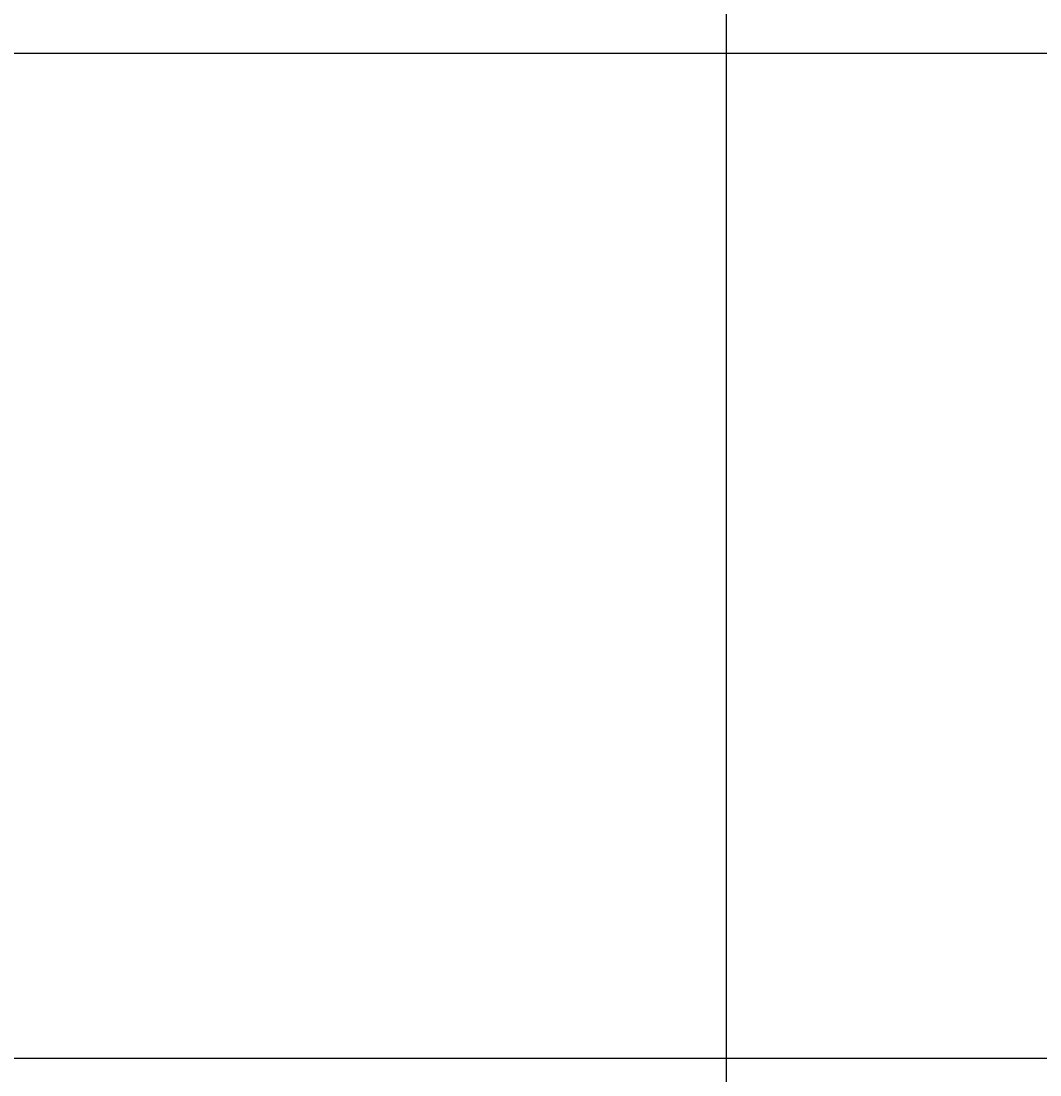
# Model space of a CAD drawing. Units: inches. Extents: x 35362 to 73946, y 43607 to 67532.
# Tile 68 of 134: x 48170 to 48464, y 48965 to 49269. Entities that reach past the tile are written whole.
import ezdxf

# ---------------------------------------------------------------- set-up
doc = ezdxf.new("R2010")
doc.units = ezdxf.units.IN
doc.header["$MEASUREMENT"] = 0
doc.layers.add('A-ANNO-DIMS', color=2, linetype='Continuous', lineweight=18)
doc.styles.get("Standard").update_dxf_attribs({"font": 'arial.ttf'})
doc.dimstyles.get("Standard").update_dxf_attribs({"dimtxt": 0.18, "dimasz": 0.18, "dimexe": 0.18, "dimexo": 0.0625, "dimgap": 0.09, "dimtad": 0, "dimtih": 1, "dimtoh": 1, "dimdec": 4, "dimzin": 0, "dimdsep": 46, "dimtxsty": 'Standard', "dimcen": 0.09, "dimadec": 0, "dimazin": 0, "dimtfac": 1, "dimtdec": 4, "dimtofl": 0, "dimtmove": 0, "dimatfit": 3, "dimfxl": 1, "dimtolj": 1, "dimtzin": 0, "dimarcsym": 0})

# ---------------------------------------------------------------- blocks, each defined once
blk = doc.blocks.new('*D11')
at = {"layer": 'A-ANNO-DIMS', "color": 0, "lineweight": -2, "transparency": 16777216}
for p, q in [((47978.66, 56028.77), (47978.66, 43606.68)), ((53109.76, 56028.77), (53109.76, 43606.68)), ((47978.84, 43606.86), (50543.87, 43606.86)), ((53109.58, 43606.86), (50544.55, 43606.86))]:
    blk.add_line(p, q, dxfattribs=at)
at = {"layer": 'A-ANNO-DIMS', "color": 0, "transparency": 16777216}
for points in [[(47978.84, 43606.89), (47978.84, 43606.83), (47978.66, 43606.86)], [(53109.58, 43606.89), (53109.58, 43606.83), (53109.76, 43606.86)]]:
    blk.add_solid(points, dxfattribs=at)
at = {"layer": 'Defpoints', "color": 0, "transparency": 16777216}
for p in [(47978.66, 56028.84), (53109.76, 56028.84), (53109.76, 43606.86)]:
    blk.add_point(p, dxfattribs=at)
at = {"layer": 'A-ANNO-DIMS', "color": 0, "transparency": 16777216, "insert": (50544.21, 43606.86), "char_height": 0.18, "attachment_point": 5}
blk.add_mtext('\\A1;5131', dxfattribs=at)
blk = doc.blocks.new('*D13')
at = {"layer": 'A-ANNO-DIMS', "color": 0, "lineweight": -2, "transparency": 16777216}
for p, q in [((48373.49, 51694.02), (48373.49, 43606.68)), ((51029.04, 51694.02), (51029.04, 43606.68)), ((48373.67, 43606.86), (49700.8, 43606.86)), ((51028.86, 43606.86), (49701.73, 43606.86))]:
    blk.add_line(p, q, dxfattribs=at)
at = {"layer": 'A-ANNO-DIMS', "color": 0, "transparency": 16777216}
for points in [[(48373.67, 43606.89), (48373.67, 43606.83), (48373.49, 43606.86)], [(51028.86, 43606.89), (51028.86, 43606.83), (51029.04, 43606.86)]]:
    blk.add_solid(points, dxfattribs=at)
at = {"layer": 'Defpoints', "color": 0, "transparency": 16777216}
for p in [(48373.49, 51694.09), (51029.04, 51694.09), (51029.04, 43606.86)]:
    blk.add_point(p, dxfattribs=at)
at = {"layer": 'A-ANNO-DIMS', "color": 0, "transparency": 16777216, "insert": (49701.27, 43606.86), "char_height": 0.18, "attachment_point": 5}
blk.add_mtext('\\A1;2655.6', dxfattribs=at)
blk = doc.blocks.new('*D27')
at = {"layer": 'A-ANNO-DIMS', "color": 0, "lineweight": -2, "transparency": 16777216}
for p, q in [((47978.66, 56028.77), (47978.66, 43606.68)), ((48373.49, 53428.96), (48373.49, 43606.68)), ((47978.84, 43606.86), (48175.68, 43606.86)), ((48373.31, 43606.86), (48176.47, 43606.86))]:
    blk.add_line(p, q, dxfattribs=at)
at = {"layer": 'A-ANNO-DIMS', "color": 0, "transparency": 16777216}
for points in [[(47978.84, 43606.89), (47978.84, 43606.83), (47978.66, 43606.86)], [(48373.31, 43606.89), (48373.31, 43606.83), (48373.49, 43606.86)]]:
    blk.add_solid(points, dxfattribs=at)
at = {"layer": 'Defpoints', "color": 0, "transparency": 16777216}
for p in [(47978.66, 56028.84), (48373.49, 53429.02), (48373.49, 43606.86)]:
    blk.add_point(p, dxfattribs=at)
at = {"layer": 'A-ANNO-DIMS', "color": 0, "transparency": 16777216, "insert": (48176.08, 43606.86), "char_height": 0.18, "attachment_point": 5}
blk.add_mtext('\\A1;394.8', dxfattribs=at)
blk = doc.blocks.new('*D67')
at = {"layer": 'A-ANNO-DIMS', "color": 0, "lineweight": -2, "transparency": 16777216}
for p, q in [((56873.54, 53351.53), (35361.77, 53351.53)), ((35361.95, 53351.35), (35361.95, 49400.89)), ((35361.95, 45450.07), (35361.95, 49400.53)), ((53793.58, 45449.89), (35361.77, 45449.89))]:
    blk.add_line(p, q, dxfattribs=at)
at = {"layer": 'A-ANNO-DIMS', "color": 0, "transparency": 16777216}
for points in [[(35361.92, 53351.35), (35361.98, 53351.35), (35361.95, 53351.53)], [(35361.92, 45450.07), (35361.98, 45450.07), (35361.95, 45449.89)]]:
    blk.add_solid(points, dxfattribs=at)
at = {"layer": 'Defpoints', "color": 0, "transparency": 16777216}
for p in [(35361.95, 53351.53), (56873.6, 53351.53), (53793.64, 45449.89)]:
    blk.add_point(p, dxfattribs=at)
at = {"layer": 'A-ANNO-DIMS', "color": 0, "transparency": 16777216, "insert": (35361.95, 49400.71), "char_height": 0.18, "attachment_point": 5}
blk.add_mtext('\\A1;7901.6', dxfattribs=at)
blk = doc.blocks.new('*D84')
at = {"layer": 'A-ANNO-DIMS', "color": 0, "lineweight": -2, "transparency": 16777216}
for p, q in [((55540.23, 49259.94), (35361.77, 49259.94)), ((35361.95, 49259.76), (35361.95, 49115.14)), ((35361.95, 48970.16), (35361.95, 49114.78)), ((55540.23, 48969.98), (35361.77, 48969.98))]:
    blk.add_line(p, q, dxfattribs=at)
at = {"layer": 'A-ANNO-DIMS', "color": 0, "transparency": 16777216}
for points in [[(35361.92, 49259.76), (35361.98, 49259.76), (35361.95, 49259.94)], [(35361.92, 48970.16), (35361.98, 48970.16), (35361.95, 48969.98)]]:
    blk.add_solid(points, dxfattribs=at)
at = {"layer": 'Defpoints', "color": 0, "transparency": 16777216}
for p in [(35361.95, 49259.94), (55540.3, 49259.94), (55540.3, 48969.98)]:
    blk.add_point(p, dxfattribs=at)
at = {"layer": 'A-ANNO-DIMS', "color": 0, "transparency": 16777216, "insert": (35361.95, 49114.96), "char_height": 0.18, "attachment_point": 5}
blk.add_mtext('\\A1;289.96', dxfattribs=at)
blk = doc.blocks.new('*D86')
at = {"layer": 'A-ANNO-DIMS', "color": 0, "lineweight": -2, "transparency": 16777216}
for p, q in [((51285.53, 49320.08), (35361.77, 49320.08)), ((35361.95, 49319.9), (35361.95, 49120.26)), ((35361.95, 48920.26), (35361.95, 49119.9)), ((51285.53, 48920.08), (35361.77, 48920.08))]:
    blk.add_line(p, q, dxfattribs=at)
at = {"layer": 'A-ANNO-DIMS', "color": 0, "transparency": 16777216}
for points in [[(35361.92, 49319.9), (35361.98, 49319.9), (35361.95, 49320.08)], [(35361.92, 48920.26), (35361.98, 48920.26), (35361.95, 48920.08)]]:
    blk.add_solid(points, dxfattribs=at)
at = {"layer": 'Defpoints', "color": 0, "transparency": 16777216}
for p in [(35361.95, 49320.08), (51285.59, 49320.08), (51285.59, 48920.08)]:
    blk.add_point(p, dxfattribs=at)
at = {"layer": 'A-ANNO-DIMS', "color": 0, "transparency": 16777216, "insert": (35361.95, 49120.08), "char_height": 0.18, "attachment_point": 5}
blk.add_mtext('\\A1;400.0', dxfattribs=at)

msp = doc.modelspace()

# ---------------------------------------------------------------- dimensions: what is measured, and where the dimension line sits
at = {"layer": 'A-ANNO-DIMS'}
for base, p1, p2, override, picture, middle in [((53109.76, 43606.859), (47978.665, 56028.836), (53109.76, 56028.836), {"dimdec": 0, "dimlfac": 1, "dimrnd": 0, "dimzin": 0, "dimdsep": 46, "dimlunit": 2}, '*D11', (50544.212, 43606.859)), ((48373.492, 43606.859), (47978.665, 56028.836), (48373.492, 53429.019), {"dimdec": 1, "dimlfac": 1, "dimrnd": 0, "dimzin": 0, "dimdsep": 46, "dimlunit": 2}, '*D27', (48176.078, 43606.859)), ((51029.043, 43606.859), (48373.492, 51694.087), (51029.043, 51694.087), {"dimdec": 1, "dimlfac": 1, "dimrnd": 0, "dimzin": 0, "dimdsep": 46, "dimlunit": 2}, '*D13', (49701.267, 43606.859))]:
    dim = msp.add_linear_dim(base=base, p1=p1, p2=p2, dimstyle='Standard', override=override, dxfattribs=at)
    dim.commit()
    dim.dimension.update_dxf_attribs({"geometry": picture, "text_midpoint": middle})
for base, p1, p2, override, picture, middle in [((35361.949, 53351.529), (53793.638, 45449.894), (56873.602, 53351.529), {"dimdec": 1, "dimlfac": 1, "dimrnd": 0, "dimzin": 0, "dimdsep": 46, "dimlunit": 2}, '*D67', (35361.949, 49400.712)), ((35361.949, 49320.079), (51285.595, 48920.079), (51285.595, 49320.079), {"dimdec": 1, "dimlfac": 1, "dimrnd": 0, "dimzin": 0, "dimdsep": 46, "dimlunit": 2}, '*D86', (35361.949, 49120.079)), ((35361.9491, 49259.9353), (55540.2972, 48969.9796), (55540.2972, 49259.9353), {"dimdec": 2, "dimlfac": 1, "dimrnd": 0, "dimzin": 0, "dimdsep": 46, "dimlunit": 2}, '*D84', (35361.9491, 49114.9575))]:
    dim = msp.add_linear_dim(base=base, p1=p1, p2=p2, angle=90, dimstyle='Standard', override=override, dxfattribs=at)
    dim.commit()
    dim.dimension.update_dxf_attribs({"geometry": picture, "text_midpoint": middle})

doc.saveas('drawing.dxf')
